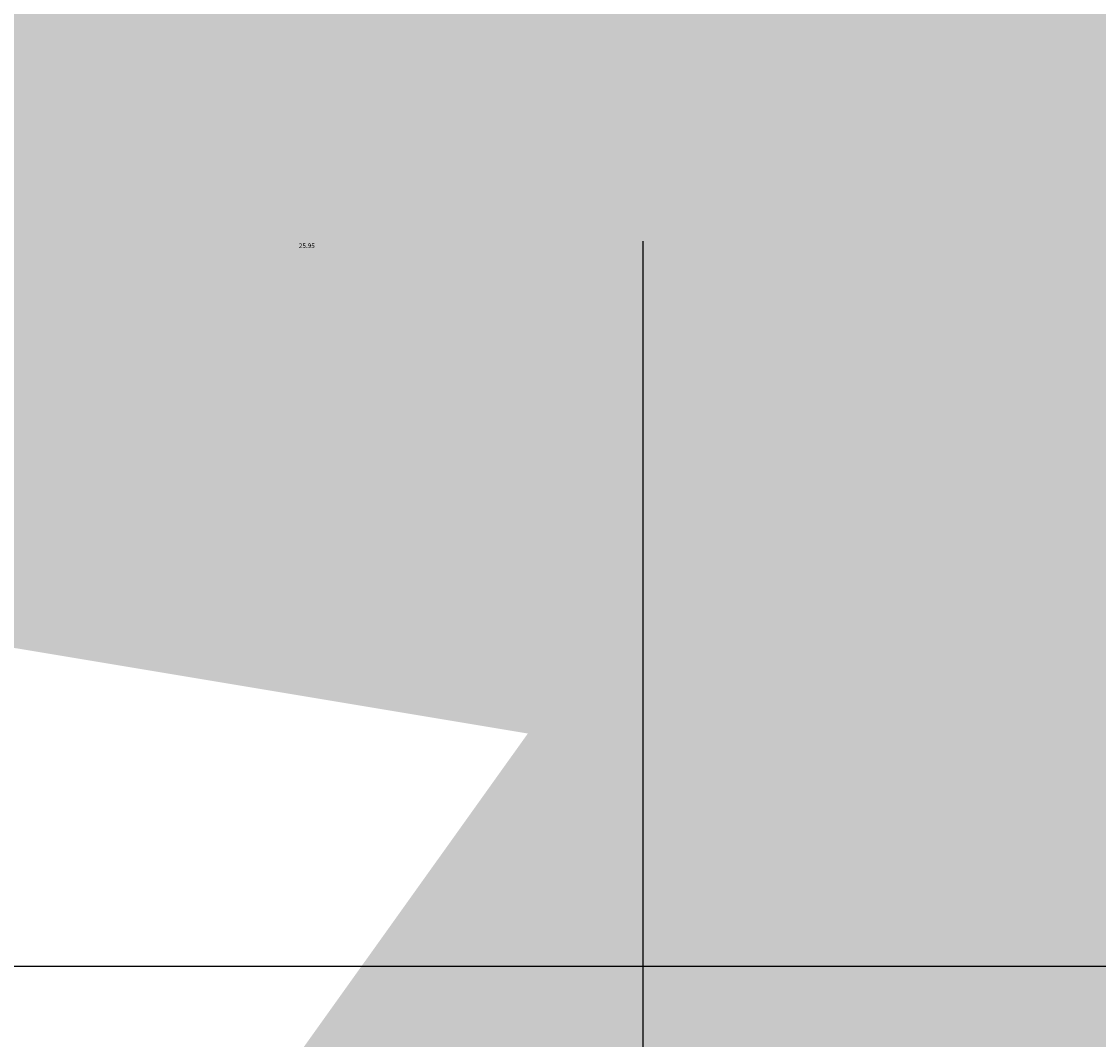
# Model space of a CAD drawing. Units: millimetres. Extents: x -22994 to 29398, y -19990 to 20176.
# Tile 119 of 135: x 204 to 245, y 174 to 213. Entities that reach past the tile are written whole.
import ezdxf

# ---------------------------------------------------------------- set-up
doc = ezdxf.new("R2010")
doc.units = ezdxf.units.MM
doc.header["$MEASUREMENT"] = 0
doc.layers.add('M-DIMS', color=2, linetype='Continuous', lineweight=18)
doc.styles.get("Standard").update_dxf_attribs({"font": 'arial.ttf'})
doc.dimstyles.get("Standard").update_dxf_attribs({"dimtxt": 0.18, "dimasz": 10000, "dimexe": 0.18, "dimexo": 0.0625, "dimgap": 0.09, "dimtad": 0, "dimtih": 1, "dimtoh": 1, "dimdec": 0, "dimzin": 0, "dimdsep": 46, "dimtxsty": 'Standard', "dimcen": 0.09, "dimadec": 0, "dimazin": 0, "dimtfac": 1, "dimtdec": 0, "dimtofl": 0, "dimtmove": 0, "dimatfit": 3, "dimfxl": 1, "dimtolj": 1, "dimtzin": 0, "dimlwd": 30, "dimarcsym": 0})

# ---------------------------------------------------------------- blocks, each defined once
blk = doc.blocks.new('*D2')
at = {"layer": 'Defpoints', "color": 0, "transparency": 16777216}
for p in [(6.677, 10.271), (290.852, 10.271), (290.852, -5.079)]:
    blk.add_point(p, dxfattribs=at)
at = {"layer": 'M-DIMS', "color": 0, "lineweight": -2, "transparency": 16777216}
for p, q in [((6.677, 10.209), (6.677, -5.259)), ((290.852, 10.209), (290.852, -5.259))]:
    blk.add_line(p, q, dxfattribs=at)
at = {"layer": 'M-DIMS', "color": 0, "lineweight": 30, "transparency": 16777216}
for p, q in [((-9993.323, -5.079), (-19993.323, -5.079)), ((10290.852, -5.079), (20290.852, -5.079))]:
    blk.add_line(p, q, dxfattribs=at)
at = {"layer": 'M-DIMS', "color": 0, "transparency": 16777216}
for points in [[(-9993.323, 1661.588), (-9993.323, -1671.745), (6.677, -5.079)], [(10290.852, 1661.588), (10290.852, -1671.745), (290.852, -5.079)]]:
    blk.add_solid(points, dxfattribs=at)
at = {"layer": 'M-DIMS', "color": 0, "transparency": 16777216, "insert": (148.765, -5.079), "char_height": 0.18, "attachment_point": 5}
blk.add_mtext('\\A1;284.2', dxfattribs=at)
blk = doc.blocks.new('*D3')
at = {"layer": 'Defpoints', "color": 0, "transparency": 16777216}
for p in [(110.265, 204.165), (110.265, 176.366), (95.833, 127.967)]:
    blk.add_point(p, dxfattribs=at)
at = {"layer": 'M-DIMS', "color": 0, "lineweight": 30, "transparency": 16777216}
for p, q in [((-9904.167, 204.165), (-19904.167, 204.165)), ((10110.265, 204.165), (20110.265, 204.165))]:
    blk.add_line(p, q, dxfattribs=at)
at = {"layer": 'M-DIMS', "color": 0, "lineweight": -2, "transparency": 16777216}
for p, q in [((95.833, 128.03), (95.833, 204.345)), ((110.265, 176.429), (110.265, 204.345))]:
    blk.add_line(p, q, dxfattribs=at)
at = {"layer": 'M-DIMS', "color": 0, "transparency": 16777216}
for points in [[(-9904.167, 1870.832), (-9904.167, -1462.501), (95.833, 204.165)], [(10110.265, 1870.832), (10110.265, -1462.501), (110.265, 204.165)]]:
    blk.add_solid(points, dxfattribs=at)
at = {"layer": 'M-DIMS', "color": 0, "transparency": 16777216, "insert": (103.049, 204.165), "char_height": 0.18, "attachment_point": 5}
blk.add_mtext('\\A1;14.432', dxfattribs=at)
blk = doc.blocks.new('*D4')
at = {"layer": 'Defpoints', "color": 0, "transparency": 16777216}
for p in [(116.265, 204.165), (110.265, 176.366), (116.265, 176.366)]:
    blk.add_point(p, dxfattribs=at)
at = {"layer": 'M-DIMS', "color": 0, "lineweight": 30, "transparency": 16777216}
for p, q in [((-9889.735, 204.165), (-19889.735, 204.165)), ((10116.265, 204.165), (20116.265, 204.165))]:
    blk.add_line(p, q, dxfattribs=at)
at = {"layer": 'M-DIMS', "color": 0, "lineweight": -2, "transparency": 16777216}
for p, q in [((110.265, 176.429), (110.265, 204.345)), ((116.265, 176.429), (116.265, 204.345))]:
    blk.add_line(p, q, dxfattribs=at)
at = {"layer": 'M-DIMS', "color": 0, "transparency": 16777216}
for points in [[(-9889.735, 1870.832), (-9889.735, -1462.501), (110.265, 204.165)], [(10116.265, 1870.832), (10116.265, -1462.501), (116.265, 204.165)]]:
    blk.add_solid(points, dxfattribs=at)
at = {"layer": 'M-DIMS', "color": 0, "transparency": 16777216, "insert": (113.265, 204.165), "char_height": 0.18, "attachment_point": 5}
blk.add_mtext('\\A1;6', dxfattribs=at)
blk = doc.blocks.new('*D5')
at = {"layer": 'Defpoints', "color": 0, "transparency": 16777216}
for p in [(181.265, 204.165), (116.265, 176.366), (181.265, 176.366)]:
    blk.add_point(p, dxfattribs=at)
at = {"layer": 'M-DIMS', "color": 0, "lineweight": 30, "transparency": 16777216}
for p, q in [((-9883.735, 204.165), (-19883.735, 204.165)), ((10181.265, 204.165), (20181.265, 204.165))]:
    blk.add_line(p, q, dxfattribs=at)
at = {"layer": 'M-DIMS', "color": 0, "lineweight": -2, "transparency": 16777216}
for p, q in [((116.265, 176.429), (116.265, 204.345)), ((181.265, 176.429), (181.265, 204.345))]:
    blk.add_line(p, q, dxfattribs=at)
at = {"layer": 'M-DIMS', "color": 0, "transparency": 16777216}
for points in [[(-9883.735, 1870.832), (-9883.735, -1462.501), (116.265, 204.165)], [(10181.265, 1870.832), (10181.265, -1462.501), (181.265, 204.165)]]:
    blk.add_solid(points, dxfattribs=at)
at = {"layer": 'M-DIMS', "color": 0, "transparency": 16777216, "insert": (148.765, 204.165), "char_height": 0.18, "attachment_point": 5}
blk.add_mtext('\\A1;65', dxfattribs=at)
blk = doc.blocks.new('*D6')
at = {"layer": 'Defpoints', "color": 0, "transparency": 16777216}
for p in [(187.265, 204.165), (181.265, 176.366), (187.265, 176.366)]:
    blk.add_point(p, dxfattribs=at)
at = {"layer": 'M-DIMS', "color": 0, "lineweight": 30, "transparency": 16777216}
for p, q in [((-9818.735, 204.165), (-19818.735, 204.165)), ((10187.265, 204.165), (20187.265, 204.165))]:
    blk.add_line(p, q, dxfattribs=at)
at = {"layer": 'M-DIMS', "color": 0, "lineweight": -2, "transparency": 16777216}
for p, q in [((181.265, 176.429), (181.265, 204.345)), ((187.265, 176.429), (187.265, 204.345))]:
    blk.add_line(p, q, dxfattribs=at)
at = {"layer": 'M-DIMS', "color": 0, "transparency": 16777216}
for points in [[(-9818.735, 1870.832), (-9818.735, -1462.501), (181.265, 204.165)], [(10187.265, 1870.832), (10187.265, -1462.501), (187.265, 204.165)]]:
    blk.add_solid(points, dxfattribs=at)
at = {"layer": 'M-DIMS', "color": 0, "transparency": 16777216, "insert": (184.265, 204.165), "char_height": 0.18, "attachment_point": 5}
blk.add_mtext('\\A1;6', dxfattribs=at)
blk = doc.blocks.new('*D7')
at = {"layer": 'Defpoints', "color": 0, "transparency": 16777216}
for p in [(201.697, 204.165), (187.265, 176.366), (201.697, 127.967)]:
    blk.add_point(p, dxfattribs=at)
at = {"layer": 'M-DIMS', "color": 0, "lineweight": 30, "transparency": 16777216}
for p, q in [((-9812.735, 204.165), (-19812.735, 204.165)), ((10201.697, 204.165), (20201.697, 204.165))]:
    blk.add_line(p, q, dxfattribs=at)
at = {"layer": 'M-DIMS', "color": 0, "lineweight": -2, "transparency": 16777216}
for p, q in [((187.265, 176.429), (187.265, 204.345)), ((201.697, 128.03), (201.697, 204.345))]:
    blk.add_line(p, q, dxfattribs=at)
at = {"layer": 'M-DIMS', "color": 0, "transparency": 16777216}
for points in [[(-9812.735, 1870.832), (-9812.735, -1462.501), (187.265, 204.165)], [(10201.697, 1870.832), (10201.697, -1462.501), (201.697, 204.165)]]:
    blk.add_solid(points, dxfattribs=at)
at = {"layer": 'M-DIMS', "color": 0, "transparency": 16777216, "insert": (194.481, 204.165), "char_height": 0.18, "attachment_point": 5}
blk.add_mtext('\\A1;14.432', dxfattribs=at)
blk = doc.blocks.new('*D8')
at = {"layer": 'Defpoints', "color": 0, "transparency": 16777216}
for p in [(227.648, 204.165), (227.648, 146.73), (201.697, 127.967)]:
    blk.add_point(p, dxfattribs=at)
at = {"layer": 'M-DIMS', "color": 0, "lineweight": 30, "transparency": 16777216}
for p, q in [((-9798.303, 204.165), (-19798.303, 204.165)), ((10227.648, 204.165), (20227.648, 204.165))]:
    blk.add_line(p, q, dxfattribs=at)
at = {"layer": 'M-DIMS', "color": 0, "lineweight": -2, "transparency": 16777216}
for p, q in [((201.697, 128.03), (201.697, 204.345)), ((227.648, 146.792), (227.648, 204.345))]:
    blk.add_line(p, q, dxfattribs=at)
at = {"layer": 'M-DIMS', "color": 0, "transparency": 16777216}
for points in [[(-9798.303, 1870.832), (-9798.303, -1462.501), (201.697, 204.165)], [(10227.648, 1870.832), (10227.648, -1462.501), (227.648, 204.165)]]:
    blk.add_solid(points, dxfattribs=at)
at = {"layer": 'M-DIMS', "color": 0, "transparency": 16777216, "insert": (214.673, 204.165), "char_height": 0.18, "attachment_point": 5}
blk.add_mtext('\\A1;25.95', dxfattribs=at)
blk = doc.blocks.new('*D9')
at = {"layer": 'Defpoints', "color": 0, "transparency": 16777216}
for p in [(187.265, 176.366), (306.202, 176.366), (290.852, 10.271)]:
    blk.add_point(p, dxfattribs=at)
at = {"layer": 'M-DIMS', "color": 0, "lineweight": 30, "transparency": 16777216}
for p, q in [((306.202, 10176.366), (306.202, 20176.366)), ((306.202, -9989.729), (306.202, -19989.729))]:
    blk.add_line(p, q, dxfattribs=at)
at = {"layer": 'M-DIMS', "color": 0, "lineweight": -2, "transparency": 16777216}
for p, q in [((187.327, 176.366), (306.382, 176.366)), ((290.915, 10.271), (306.382, 10.271))]:
    blk.add_line(p, q, dxfattribs=at)
at = {"layer": 'M-DIMS', "color": 0, "transparency": 16777216}
for points in [[(-1360.465, 10176.366), (1972.869, 10176.366), (306.202, 176.366)], [(-1360.465, -9989.729), (1972.869, -9989.729), (306.202, 10.271)]]:
    blk.add_solid(points, dxfattribs=at)
at = {"layer": 'M-DIMS', "color": 0, "transparency": 16777216, "insert": (306.202, 93.319), "char_height": 0.18, "attachment_point": 5}
blk.add_mtext('\\A1;166.1', dxfattribs=at)
blk = doc.blocks.new('*D10')
at = {"layer": 'Defpoints', "color": 0, "transparency": 16777216}
for p in [(125.65, 136.071), (133.346, 136.071), (133.346, -5.079)]:
    blk.add_point(p, dxfattribs=at)
at = {"layer": 'M-DIMS', "color": 0, "lineweight": -2, "transparency": 16777216}
for p, q in [((125.65, 136.009), (125.65, -5.259)), ((133.346, 136.009), (133.346, -5.259))]:
    blk.add_line(p, q, dxfattribs=at)
at = {"layer": 'M-DIMS', "color": 0, "lineweight": 30, "transparency": 16777216}
for p, q in [((-9874.35, -5.079), (-19874.35, -5.079)), ((10133.346, -5.079), (20133.346, -5.079))]:
    blk.add_line(p, q, dxfattribs=at)
at = {"layer": 'M-DIMS', "color": 0, "transparency": 16777216}
for points in [[(-9874.35, 1661.588), (-9874.35, -1671.745), (125.65, -5.079)], [(10133.346, 1661.588), (10133.346, -1671.745), (133.346, -5.079)]]:
    blk.add_solid(points, dxfattribs=at)
at = {"layer": 'M-DIMS', "color": 0, "transparency": 16777216, "insert": (129.498, -5.079), "char_height": 0.18, "attachment_point": 5}
blk.add_mtext('\\A1;7.696', dxfattribs=at)
blk = doc.blocks.new('*D11')
at = {"layer": 'Defpoints', "color": 0, "transparency": 16777216}
for p in [(133.346, 136.071), (135.65, 136.071), (135.65, -5.079)]:
    blk.add_point(p, dxfattribs=at)
at = {"layer": 'M-DIMS', "color": 0, "lineweight": -2, "transparency": 16777216}
for p, q in [((133.346, 136.009), (133.346, -5.259)), ((135.65, 136.009), (135.65, -5.259))]:
    blk.add_line(p, q, dxfattribs=at)
at = {"layer": 'M-DIMS', "color": 0, "lineweight": 30, "transparency": 16777216}
for p, q in [((-9866.654, -5.079), (-19866.654, -5.079)), ((10135.65, -5.079), (20135.65, -5.079))]:
    blk.add_line(p, q, dxfattribs=at)
at = {"layer": 'M-DIMS', "color": 0, "transparency": 16777216}
for points in [[(-9866.654, 1661.588), (-9866.654, -1671.745), (133.346, -5.079)], [(10135.65, 1661.588), (10135.65, -1671.745), (135.65, -5.079)]]:
    blk.add_solid(points, dxfattribs=at)
at = {"layer": 'M-DIMS', "color": 0, "transparency": 16777216, "insert": (134.498, -5.079), "char_height": 0.18, "attachment_point": 5}
blk.add_mtext('\\A1;2.304', dxfattribs=at)
blk = doc.blocks.new('*D12')
at = {"layer": 'Defpoints', "color": 0, "transparency": 16777216}
for p in [(135.65, 136.071), (145.65, 136.071), (145.65, -5.079)]:
    blk.add_point(p, dxfattribs=at)
at = {"layer": 'M-DIMS', "color": 0, "lineweight": -2, "transparency": 16777216}
for p, q in [((135.65, 136.009), (135.65, -5.259)), ((145.65, 136.009), (145.65, -5.259))]:
    blk.add_line(p, q, dxfattribs=at)
at = {"layer": 'M-DIMS', "color": 0, "lineweight": 30, "transparency": 16777216}
for p, q in [((-9864.35, -5.079), (-19864.35, -5.079)), ((10145.65, -5.079), (20145.65, -5.079))]:
    blk.add_line(p, q, dxfattribs=at)
at = {"layer": 'M-DIMS', "color": 0, "transparency": 16777216}
for points in [[(-9864.35, 1661.588), (-9864.35, -1671.745), (135.65, -5.079)], [(10145.65, 1661.588), (10145.65, -1671.745), (145.65, -5.079)]]:
    blk.add_solid(points, dxfattribs=at)
at = {"layer": 'M-DIMS', "color": 0, "transparency": 16777216, "insert": (140.65, -5.079), "char_height": 0.18, "attachment_point": 5}
blk.add_mtext('\\A1;10', dxfattribs=at)
blk = doc.blocks.new('*D13')
at = {"layer": 'Defpoints', "color": 0, "transparency": 16777216}
for p in [(145.65, 136.071), (155.65, 136.071), (155.65, -5.079)]:
    blk.add_point(p, dxfattribs=at)
at = {"layer": 'M-DIMS', "color": 0, "lineweight": -2, "transparency": 16777216}
for p, q in [((145.65, 136.009), (145.65, -5.259)), ((155.65, 136.009), (155.65, -5.259))]:
    blk.add_line(p, q, dxfattribs=at)
at = {"layer": 'M-DIMS', "color": 0, "lineweight": 30, "transparency": 16777216}
for p, q in [((-9854.35, -5.079), (-19854.35, -5.079)), ((10155.65, -5.079), (20155.65, -5.079))]:
    blk.add_line(p, q, dxfattribs=at)
at = {"layer": 'M-DIMS', "color": 0, "transparency": 16777216}
for points in [[(-9854.35, 1661.588), (-9854.35, -1671.745), (145.65, -5.079)], [(10155.65, 1661.588), (10155.65, -1671.745), (155.65, -5.079)]]:
    blk.add_solid(points, dxfattribs=at)
at = {"layer": 'M-DIMS', "color": 0, "transparency": 16777216, "insert": (150.65, -5.079), "char_height": 0.18, "attachment_point": 5}
blk.add_mtext('\\A1;10', dxfattribs=at)
blk = doc.blocks.new('*D14')
at = {"layer": 'Defpoints', "color": 0, "transparency": 16777216}
for p in [(155.65, 136.071), (165.65, 136.071), (165.65, -5.079)]:
    blk.add_point(p, dxfattribs=at)
at = {"layer": 'M-DIMS', "color": 0, "lineweight": -2, "transparency": 16777216}
for p, q in [((155.65, 136.009), (155.65, -5.259)), ((165.65, 136.009), (165.65, -5.259))]:
    blk.add_line(p, q, dxfattribs=at)
at = {"layer": 'M-DIMS', "color": 0, "lineweight": 30, "transparency": 16777216}
for p, q in [((-9844.35, -5.079), (-19844.35, -5.079)), ((10165.65, -5.079), (20165.65, -5.079))]:
    blk.add_line(p, q, dxfattribs=at)
at = {"layer": 'M-DIMS', "color": 0, "transparency": 16777216}
for points in [[(-9844.35, 1661.588), (-9844.35, -1671.745), (155.65, -5.079)], [(10165.65, 1661.588), (10165.65, -1671.745), (165.65, -5.079)]]:
    blk.add_solid(points, dxfattribs=at)
at = {"layer": 'M-DIMS', "color": 0, "transparency": 16777216, "insert": (160.65, -5.079), "char_height": 0.18, "attachment_point": 5}
blk.add_mtext('\\A1;10', dxfattribs=at)
blk = doc.blocks.new('*D15')
at = {"layer": 'Defpoints', "color": 0, "transparency": 16777216}
for p in [(173.346, 154.788), (173.346, 136.071), (306.202, 136.071)]:
    blk.add_point(p, dxfattribs=at)
at = {"layer": 'M-DIMS', "color": 0, "lineweight": 30, "transparency": 16777216}
for p, q in [((306.202, 10154.788), (306.202, 20154.788)), ((306.202, -9863.929), (306.202, -19863.929))]:
    blk.add_line(p, q, dxfattribs=at)
at = {"layer": 'M-DIMS', "color": 0, "lineweight": -2, "transparency": 16777216}
for p, q in [((173.408, 154.788), (306.382, 154.788)), ((173.408, 136.071), (306.382, 136.071))]:
    blk.add_line(p, q, dxfattribs=at)
at = {"layer": 'M-DIMS', "color": 0, "transparency": 16777216}
for points in [[(-1360.465, 10154.788), (1972.869, 10154.788), (306.202, 154.788)], [(-1360.465, -9863.929), (1972.869, -9863.929), (306.202, 136.071)]]:
    blk.add_solid(points, dxfattribs=at)
at = {"layer": 'M-DIMS', "color": 0, "transparency": 16777216, "insert": (306.202, 145.43), "char_height": 0.18, "attachment_point": 5}
blk.add_mtext('\\A1;18.717', dxfattribs=at)
blk = doc.blocks.new('*D16')
at = {"layer": 'Defpoints', "color": 0, "transparency": 16777216}
for p in [(120.17, 204.165), (110.466, 48.035), (120.17, 48.035)]:
    blk.add_point(p, dxfattribs=at)
at = {"layer": 'M-DIMS', "color": 0, "lineweight": 30, "transparency": 16777216}
for p, q in [((-9889.534, 204.165), (-19889.534, 204.165)), ((10120.17, 204.165), (20120.17, 204.165))]:
    blk.add_line(p, q, dxfattribs=at)
at = {"layer": 'M-DIMS', "color": 0, "lineweight": -2, "transparency": 16777216}
for p, q in [((110.466, 48.097), (110.466, 204.345)), ((120.17, 48.097), (120.17, 204.345))]:
    blk.add_line(p, q, dxfattribs=at)
at = {"layer": 'M-DIMS', "color": 0, "transparency": 16777216}
for points in [[(-9889.534, 1870.832), (-9889.534, -1462.501), (110.466, 204.165)], [(10120.17, 1870.832), (10120.17, -1462.501), (120.17, 204.165)]]:
    blk.add_solid(points, dxfattribs=at)
at = {"layer": 'M-DIMS', "color": 0, "transparency": 16777216, "insert": (115.318, 204.165), "char_height": 0.18, "attachment_point": 5}
blk.add_mtext('\\A1;9.704', dxfattribs=at)
blk = doc.blocks.new('*D17')
at = {"layer": 'Defpoints', "color": 0, "transparency": 16777216}
for p in [(126.17, 204.165), (120.17, 48.035), (126.17, 48.035)]:
    blk.add_point(p, dxfattribs=at)
at = {"layer": 'M-DIMS', "color": 0, "lineweight": 30, "transparency": 16777216}
for p, q in [((-9879.83, 204.165), (-19879.83, 204.165)), ((10126.17, 204.165), (20126.17, 204.165))]:
    blk.add_line(p, q, dxfattribs=at)
at = {"layer": 'M-DIMS', "color": 0, "lineweight": -2, "transparency": 16777216}
for p, q in [((120.17, 48.097), (120.17, 204.345)), ((126.17, 48.097), (126.17, 204.345))]:
    blk.add_line(p, q, dxfattribs=at)
at = {"layer": 'M-DIMS', "color": 0, "transparency": 16777216}
for points in [[(-9879.83, 1870.832), (-9879.83, -1462.501), (120.17, 204.165)], [(10126.17, 1870.832), (10126.17, -1462.501), (126.17, 204.165)]]:
    blk.add_solid(points, dxfattribs=at)
at = {"layer": 'M-DIMS', "color": 0, "transparency": 16777216, "insert": (123.17, 204.165), "char_height": 0.18, "attachment_point": 5}
blk.add_mtext('\\A1;6', dxfattribs=at)
blk = doc.blocks.new('*D18')
at = {"layer": 'Defpoints', "color": 0, "transparency": 16777216}
for p in [(132.17, 204.165), (126.17, 48.035), (132.17, 48.035)]:
    blk.add_point(p, dxfattribs=at)
at = {"layer": 'M-DIMS', "color": 0, "lineweight": 30, "transparency": 16777216}
for p, q in [((-9873.83, 204.165), (-19873.83, 204.165)), ((10132.17, 204.165), (20132.17, 204.165))]:
    blk.add_line(p, q, dxfattribs=at)
at = {"layer": 'M-DIMS', "color": 0, "lineweight": -2, "transparency": 16777216}
for p, q in [((126.17, 48.097), (126.17, 204.345)), ((132.17, 48.097), (132.17, 204.345))]:
    blk.add_line(p, q, dxfattribs=at)
at = {"layer": 'M-DIMS', "color": 0, "transparency": 16777216}
for points in [[(-9873.83, 1870.832), (-9873.83, -1462.501), (126.17, 204.165)], [(10132.17, 1870.832), (10132.17, -1462.501), (132.17, 204.165)]]:
    blk.add_solid(points, dxfattribs=at)
at = {"layer": 'M-DIMS', "color": 0, "transparency": 16777216, "insert": (129.17, 204.165), "char_height": 0.18, "attachment_point": 5}
blk.add_mtext('\\A1;6', dxfattribs=at)
blk = doc.blocks.new('*D19')
at = {"layer": 'Defpoints', "color": 0, "transparency": 16777216}
for p in [(138.17, 204.165), (132.17, 48.035), (138.17, 48.035)]:
    blk.add_point(p, dxfattribs=at)
at = {"layer": 'M-DIMS', "color": 0, "lineweight": 30, "transparency": 16777216}
for p, q in [((-9867.83, 204.165), (-19867.83, 204.165)), ((10138.17, 204.165), (20138.17, 204.165))]:
    blk.add_line(p, q, dxfattribs=at)
at = {"layer": 'M-DIMS', "color": 0, "lineweight": -2, "transparency": 16777216}
for p, q in [((132.17, 48.097), (132.17, 204.345)), ((138.17, 48.097), (138.17, 204.345))]:
    blk.add_line(p, q, dxfattribs=at)
at = {"layer": 'M-DIMS', "color": 0, "transparency": 16777216}
for points in [[(-9867.83, 1870.832), (-9867.83, -1462.501), (132.17, 204.165)], [(10138.17, 1870.832), (10138.17, -1462.501), (138.17, 204.165)]]:
    blk.add_solid(points, dxfattribs=at)
at = {"layer": 'M-DIMS', "color": 0, "transparency": 16777216, "insert": (135.17, 204.165), "char_height": 0.18, "attachment_point": 5}
blk.add_mtext('\\A1;6', dxfattribs=at)
blk = doc.blocks.new('*D20')
at = {"layer": 'Defpoints', "color": 0, "transparency": 16777216}
for p in [(144.17, 204.165), (138.17, 48.035), (144.17, 48.035)]:
    blk.add_point(p, dxfattribs=at)
at = {"layer": 'M-DIMS', "color": 0, "lineweight": 30, "transparency": 16777216}
for p, q in [((-9861.83, 204.165), (-19861.83, 204.165)), ((10144.17, 204.165), (20144.17, 204.165))]:
    blk.add_line(p, q, dxfattribs=at)
at = {"layer": 'M-DIMS', "color": 0, "lineweight": -2, "transparency": 16777216}
for p, q in [((138.17, 48.097), (138.17, 204.345)), ((144.17, 48.097), (144.17, 204.345))]:
    blk.add_line(p, q, dxfattribs=at)
at = {"layer": 'M-DIMS', "color": 0, "transparency": 16777216}
for points in [[(-9861.83, 1870.832), (-9861.83, -1462.501), (138.17, 204.165)], [(10144.17, 1870.832), (10144.17, -1462.501), (144.17, 204.165)]]:
    blk.add_solid(points, dxfattribs=at)
at = {"layer": 'M-DIMS', "color": 0, "transparency": 16777216, "insert": (141.17, 204.165), "char_height": 0.18, "attachment_point": 5}
blk.add_mtext('\\A1;6', dxfattribs=at)
blk = doc.blocks.new('*D21')
at = {"layer": 'Defpoints', "color": 0, "transparency": 16777216}
for p in [(149.116, 204.165), (144.17, 48.035), (149.116, 48.035)]:
    blk.add_point(p, dxfattribs=at)
at = {"layer": 'M-DIMS', "color": 0, "lineweight": 30, "transparency": 16777216}
for p, q in [((-9855.83, 204.165), (-19855.83, 204.165)), ((10149.116, 204.165), (20149.116, 204.165))]:
    blk.add_line(p, q, dxfattribs=at)
at = {"layer": 'M-DIMS', "color": 0, "lineweight": -2, "transparency": 16777216}
for p, q in [((144.17, 48.097), (144.17, 204.345)), ((149.116, 48.097), (149.116, 204.345))]:
    blk.add_line(p, q, dxfattribs=at)
at = {"layer": 'M-DIMS', "color": 0, "transparency": 16777216}
for points in [[(-9855.83, 1870.832), (-9855.83, -1462.501), (144.17, 204.165)], [(10149.116, 1870.832), (10149.116, -1462.501), (149.116, 204.165)]]:
    blk.add_solid(points, dxfattribs=at)
at = {"layer": 'M-DIMS', "color": 0, "transparency": 16777216, "insert": (146.643, 204.165), "char_height": 0.18, "attachment_point": 5}
blk.add_mtext('\\A1;4.945', dxfattribs=at)
blk = doc.blocks.new('*D22')
at = {"layer": 'Defpoints', "color": 0, "transparency": 16777216}
for p in [(149.116, 30.99), (155.116, 30.99), (155.116, -5.079)]:
    blk.add_point(p, dxfattribs=at)
at = {"layer": 'M-DIMS', "color": 0, "lineweight": -2, "transparency": 16777216}
for p, q in [((149.116, 30.927), (149.116, -5.259)), ((155.116, 30.927), (155.116, -5.259))]:
    blk.add_line(p, q, dxfattribs=at)
at = {"layer": 'M-DIMS', "color": 0, "lineweight": 30, "transparency": 16777216}
for p, q in [((-9850.884, -5.079), (-19850.884, -5.079)), ((10155.116, -5.079), (20155.116, -5.079))]:
    blk.add_line(p, q, dxfattribs=at)
at = {"layer": 'M-DIMS', "color": 0, "transparency": 16777216}
for points in [[(-9850.884, 1661.588), (-9850.884, -1671.745), (149.116, -5.079)], [(10155.116, 1661.588), (10155.116, -1671.745), (155.116, -5.079)]]:
    blk.add_solid(points, dxfattribs=at)
at = {"layer": 'M-DIMS', "color": 0, "transparency": 16777216, "insert": (152.116, -5.079), "char_height": 0.18, "attachment_point": 5}
blk.add_mtext('\\A1;6', dxfattribs=at)
blk = doc.blocks.new('*D23')
at = {"layer": 'Defpoints', "color": 0, "transparency": 16777216}
for p in [(155.116, 30.99), (161.116, 30.99), (161.116, -5.079)]:
    blk.add_point(p, dxfattribs=at)
at = {"layer": 'M-DIMS', "color": 0, "lineweight": -2, "transparency": 16777216}
for p, q in [((155.116, 30.927), (155.116, -5.259)), ((161.116, 30.927), (161.116, -5.259))]:
    blk.add_line(p, q, dxfattribs=at)
at = {"layer": 'M-DIMS', "color": 0, "lineweight": 30, "transparency": 16777216}
for p, q in [((-9844.884, -5.079), (-19844.884, -5.079)), ((10161.116, -5.079), (20161.116, -5.079))]:
    blk.add_line(p, q, dxfattribs=at)
at = {"layer": 'M-DIMS', "color": 0, "transparency": 16777216}
for points in [[(-9844.884, 1661.588), (-9844.884, -1671.745), (155.116, -5.079)], [(10161.116, 1661.588), (10161.116, -1671.745), (161.116, -5.079)]]:
    blk.add_solid(points, dxfattribs=at)
at = {"layer": 'M-DIMS', "color": 0, "transparency": 16777216, "insert": (158.116, -5.079), "char_height": 0.18, "attachment_point": 5}
blk.add_mtext('\\A1;6', dxfattribs=at)
blk = doc.blocks.new('*D24')
at = {"layer": 'Defpoints', "color": 0, "transparency": 16777216}
for p in [(161.116, 30.99), (166.439, 30.99), (166.439, -5.079)]:
    blk.add_point(p, dxfattribs=at)
at = {"layer": 'M-DIMS', "color": 0, "lineweight": -2, "transparency": 16777216}
for p, q in [((161.116, 30.927), (161.116, -5.259)), ((166.439, 30.927), (166.439, -5.259))]:
    blk.add_line(p, q, dxfattribs=at)
at = {"layer": 'M-DIMS', "color": 0, "lineweight": 30, "transparency": 16777216}
for p, q in [((-9838.884, -5.079), (-19838.884, -5.079)), ((10166.439, -5.079), (20166.439, -5.079))]:
    blk.add_line(p, q, dxfattribs=at)
at = {"layer": 'M-DIMS', "color": 0, "transparency": 16777216}
for points in [[(-9838.884, 1661.588), (-9838.884, -1671.745), (161.116, -5.079)], [(10166.439, 1661.588), (10166.439, -1671.745), (166.439, -5.079)]]:
    blk.add_solid(points, dxfattribs=at)
at = {"layer": 'M-DIMS', "color": 0, "transparency": 16777216, "insert": (163.777, -5.079), "char_height": 0.18, "attachment_point": 5}
blk.add_mtext('\\A1;5.323', dxfattribs=at)
blk = doc.blocks.new('*D25')
at = {"layer": 'Defpoints', "color": 0, "transparency": 16777216}
for p in [(166.439, 30.99), (172.439, 30.99), (172.439, -5.079)]:
    blk.add_point(p, dxfattribs=at)
at = {"layer": 'M-DIMS', "color": 0, "lineweight": -2, "transparency": 16777216}
for p, q in [((166.439, 30.927), (166.439, -5.259)), ((172.439, 30.927), (172.439, -5.259))]:
    blk.add_line(p, q, dxfattribs=at)
at = {"layer": 'M-DIMS', "color": 0, "lineweight": 30, "transparency": 16777216}
for p, q in [((-9833.561, -5.079), (-19833.561, -5.079)), ((10172.439, -5.079), (20172.439, -5.079))]:
    blk.add_line(p, q, dxfattribs=at)
at = {"layer": 'M-DIMS', "color": 0, "transparency": 16777216}
for points in [[(-9833.561, 1661.588), (-9833.561, -1671.745), (166.439, -5.079)], [(10172.439, 1661.588), (10172.439, -1671.745), (172.439, -5.079)]]:
    blk.add_solid(points, dxfattribs=at)
at = {"layer": 'M-DIMS', "color": 0, "transparency": 16777216, "insert": (169.439, -5.079), "char_height": 0.18, "attachment_point": 5}
blk.add_mtext('\\A1;6', dxfattribs=at)
blk = doc.blocks.new('*D26')
at = {"layer": 'Defpoints', "color": 0, "transparency": 16777216}
for p in [(172.439, 30.99), (178.439, 30.99), (178.439, -5.079)]:
    blk.add_point(p, dxfattribs=at)
at = {"layer": 'M-DIMS', "color": 0, "lineweight": -2, "transparency": 16777216}
for p, q in [((172.439, 30.927), (172.439, -5.259)), ((178.439, 30.927), (178.439, -5.259))]:
    blk.add_line(p, q, dxfattribs=at)
at = {"layer": 'M-DIMS', "color": 0, "lineweight": 30, "transparency": 16777216}
for p, q in [((-9827.561, -5.079), (-19827.561, -5.079)), ((10178.439, -5.079), (20178.439, -5.079))]:
    blk.add_line(p, q, dxfattribs=at)
at = {"layer": 'M-DIMS', "color": 0, "transparency": 16777216}
for points in [[(-9827.561, 1661.588), (-9827.561, -1671.745), (172.439, -5.079)], [(10178.439, 1661.588), (10178.439, -1671.745), (178.439, -5.079)]]:
    blk.add_solid(points, dxfattribs=at)
at = {"layer": 'M-DIMS', "color": 0, "transparency": 16777216, "insert": (175.439, -5.079), "char_height": 0.18, "attachment_point": 5}
blk.add_mtext('\\A1;6', dxfattribs=at)
blk = doc.blocks.new('*D27')
at = {"layer": 'Defpoints', "color": 0, "transparency": 16777216}
for p in [(178.439, 30.99), (188.117, 30.99), (188.117, -5.079)]:
    blk.add_point(p, dxfattribs=at)
at = {"layer": 'M-DIMS', "color": 0, "lineweight": -2, "transparency": 16777216}
for p, q in [((178.439, 30.927), (178.439, -5.259)), ((188.117, 30.927), (188.117, -5.259))]:
    blk.add_line(p, q, dxfattribs=at)
at = {"layer": 'M-DIMS', "color": 0, "lineweight": 30, "transparency": 16777216}
for p, q in [((-9821.561, -5.079), (-19821.561, -5.079)), ((10188.117, -5.079), (20188.117, -5.079))]:
    blk.add_line(p, q, dxfattribs=at)
at = {"layer": 'M-DIMS', "color": 0, "transparency": 16777216}
for points in [[(-9821.561, 1661.588), (-9821.561, -1671.745), (178.439, -5.079)], [(10188.117, 1661.588), (10188.117, -1671.745), (188.117, -5.079)]]:
    blk.add_solid(points, dxfattribs=at)
at = {"layer": 'M-DIMS', "color": 0, "transparency": 16777216, "insert": (183.278, -5.079), "char_height": 0.18, "attachment_point": 5}
blk.add_mtext('\\A1;9.679', dxfattribs=at)
blk = doc.blocks.new('*D28')
at = {"layer": 'Defpoints', "color": 0, "transparency": 16777216}
for p in [(188.117, 48.035), (306.202, 48.035), (188.117, 30.99)]:
    blk.add_point(p, dxfattribs=at)
at = {"layer": 'M-DIMS', "color": 0, "lineweight": 30, "transparency": 16777216}
for p, q in [((306.202, 10048.035), (306.202, 20048.035)), ((306.202, -9969.01), (306.202, -19969.01))]:
    blk.add_line(p, q, dxfattribs=at)
at = {"layer": 'M-DIMS', "color": 0, "lineweight": -2, "transparency": 16777216}
for p, q in [((188.18, 48.035), (306.382, 48.035)), ((188.18, 30.99), (306.382, 30.99))]:
    blk.add_line(p, q, dxfattribs=at)
at = {"layer": 'M-DIMS', "color": 0, "transparency": 16777216}
for points in [[(-1360.465, 10048.035), (1972.869, 10048.035), (306.202, 48.035)], [(-1360.465, -9969.01), (1972.869, -9969.01), (306.202, 30.99)]]:
    blk.add_solid(points, dxfattribs=at)
at = {"layer": 'M-DIMS', "color": 0, "transparency": 16777216, "insert": (306.202, 39.512), "char_height": 0.18, "attachment_point": 5}
blk.add_mtext('\\A1;17.045', dxfattribs=at)
blk = doc.blocks.new('*D29')
at = {"layer": 'Defpoints', "color": 0, "transparency": 16777216}
for p in [(36.801, 80.045), (64.03, 80.045)]:
    blk.add_point(p, dxfattribs=at)
at = {"layer": 'M-DIMS', "color": 0, "lineweight": -2, "transparency": 16777216}
for p, q in [((50.325, 80.045), (50.505, 80.045)), ((50.415, 79.955), (50.415, 80.135))]:
    blk.add_line(p, q, dxfattribs=at)
at = {"layer": 'M-DIMS', "color": 0, "lineweight": 30, "transparency": 16777216}
blk.add_line((20064.03, 80.03), (10064.03, 80.038), dxfattribs=at)
at = {"layer": 'M-DIMS', "color": 0, "transparency": 16777216}
blk.add_solid([(10064.031, 1746.704), (10064.028, -1586.629), (64.03, 80.045)], dxfattribs=at)
at = {"layer": 'M-DIMS', "color": 0, "transparency": 16777216, "insert": (20064.521, 80.03), "char_height": 0.18, "attachment_point": 5}
blk.add_mtext('\\A1;∅27.23', dxfattribs=at)
blk = doc.blocks.new('*D30')
at = {"layer": 'Defpoints', "color": 0, "transparency": 16777216}
for p in [(216.315, 146.729), (238.982, 146.73)]:
    blk.add_point(p, dxfattribs=at)
at = {"layer": 'M-DIMS', "color": 0, "lineweight": 30, "transparency": 16777216}
blk.add_line((20238.982, 147.496), (10238.982, 147.113), dxfattribs=at)
at = {"layer": 'M-DIMS', "color": 0, "lineweight": -2, "transparency": 16777216}
for p, q in [((227.558, 146.73), (227.738, 146.73)), ((227.648, 146.64), (227.648, 146.82))]:
    blk.add_line(p, q, dxfattribs=at)
at = {"layer": 'M-DIMS', "color": 0, "transparency": 16777216}
blk.add_solid([(10238.918, 1813.78), (10239.046, -1519.554), (238.982, 146.73)], dxfattribs=at)
at = {"layer": 'M-DIMS', "color": 0, "transparency": 16777216, "insert": (20239.544, 147.496), "char_height": 0.18, "attachment_point": 5}
blk.add_mtext('\\A1;∅22.667', dxfattribs=at)
blk = doc.blocks.new('*D31')
at = {"layer": 'Defpoints', "color": 0, "transparency": 16777216}
for p in [(223.164, 146.729), (232.133, 146.73)]:
    blk.add_point(p, dxfattribs=at)
at = {"layer": 'M-DIMS', "color": 0, "lineweight": 30, "transparency": 16777216}
blk.add_line((20232.133, 148.666), (10232.133, 147.698), dxfattribs=at)
at = {"layer": 'M-DIMS', "color": 0, "lineweight": -2, "transparency": 16777216}
for p, q in [((227.558, 146.73), (227.738, 146.73)), ((227.648, 146.64), (227.648, 146.82))]:
    blk.add_line(p, q, dxfattribs=at)
at = {"layer": 'M-DIMS', "color": 0, "transparency": 16777216}
blk.add_solid([(10231.971, 1814.364), (10232.294, -1518.969), (232.133, 146.73)], dxfattribs=at)
at = {"layer": 'M-DIMS', "color": 0, "transparency": 16777216, "insert": (20232.625, 148.666), "char_height": 0.18, "attachment_point": 5}
blk.add_mtext('\\A1;∅8.969', dxfattribs=at)
blk = doc.blocks.new('*D34')
at = {"layer": 'Defpoints', "color": 0, "transparency": 16777216}
for p in [(178.58, 122.895), (176.812, 121.128)]:
    blk.add_point(p, dxfattribs=at)
at = {"layer": 'M-DIMS', "color": 0, "lineweight": 30, "transparency": 16777216}
for p, q in [((14322.436, 14263.311), (7250.508, 7193.103)), ((24322.436, 14263.311), (14322.436, 14263.311))]:
    blk.add_line(p, q, dxfattribs=at)
at = {"layer": 'M-DIMS', "color": 0, "lineweight": -2, "transparency": 16777216}
for p, q in [((176.722, 121.128), (176.902, 121.128)), ((176.812, 121.038), (176.812, 121.218))]:
    blk.add_line(p, q, dxfattribs=at)
at = {"layer": 'M-DIMS', "color": 0, "transparency": 16777216}
blk.add_solid([(6072.14, 8371.758), (8428.876, 6014.448), (178.58, 122.895)], dxfattribs=at)
at = {"layer": 'M-DIMS', "color": 0, "transparency": 16777216, "insert": (24322.97, 14263.311), "char_height": 0.18, "attachment_point": 5}
blk.add_mtext('\\A1;6X R2.5', dxfattribs=at)
blk = doc.blocks.new('*D36')
at = {"layer": 'Defpoints', "color": 0, "transparency": 16777216}
for p in [(46.39, 31.303), (46.387, 26.593)]:
    blk.add_point(p, dxfattribs=at)
at = {"layer": 'M-DIMS', "color": 0, "lineweight": 30, "transparency": 16777216}
for p, q in [((57.15, 20031.301), (51.77, 10031.302)), ((10057.15, 20031.301), (57.15, 20031.301))]:
    blk.add_line(p, q, dxfattribs=at)
at = {"layer": 'M-DIMS', "color": 0, "lineweight": -2, "transparency": 16777216}
for p, q in [((46.299, 28.948), (46.479, 28.948)), ((46.389, 28.858), (46.389, 29.038))]:
    blk.add_line(p, q, dxfattribs=at)
at = {"layer": 'M-DIMS', "color": 0, "transparency": 16777216}
blk.add_solid([(-1614.896, 10032.199), (1718.436, 10030.405), (46.39, 31.303)], dxfattribs=at)
at = {"layer": 'M-DIMS', "color": 0, "transparency": 16777216, "insert": (10057.554, 20031.301), "char_height": 0.18, "attachment_point": 5}
blk.add_mtext('\\A1;∅4.71', dxfattribs=at)
blk = doc.blocks.new('*D37')
at = {"layer": 'Defpoints', "color": 0, "transparency": 16777216}
for p in [(54.834, 118.615), (59.494, 118.614)]:
    blk.add_point(p, dxfattribs=at)
at = {"layer": 'M-DIMS', "color": 0, "lineweight": -2, "transparency": 16777216}
for p, q in [((57.074, 118.614), (57.254, 118.614)), ((57.164, 118.524), (57.164, 118.704))]:
    blk.add_line(p, q, dxfattribs=at)
at = {"layer": 'M-DIMS', "color": 0, "lineweight": 30, "transparency": 16777216}
blk.add_line((20059.493, 116.253), (10059.494, 117.434), dxfattribs=at)
at = {"layer": 'M-DIMS', "color": 0, "transparency": 16777216}
blk.add_solid([(10059.69, 1784.1), (10059.297, -1549.233), (59.494, 118.614)], dxfattribs=at)
at = {"layer": 'M-DIMS', "color": 0, "transparency": 16777216, "insert": (20059.985, 116.253), "char_height": 0.18, "attachment_point": 5}
blk.add_mtext('\\A1;∅4.659', dxfattribs=at)

msp = doc.modelspace()

# ---------------------------------------------------------------- dimensions: what is measured, and where the dimension line sits
at = {"layer": 'M-DIMS'}
for base, p1, p2, override, picture, middle in [((306.202, 176.3662), (290.852, 10.2713), (187.2647, 176.3662), {"dimdec": 1, "dimlfac": 1, "dimrnd": 0, "dimzin": 0, "dimdsep": 46, "dimlunit": 2}, '*D9', (306.202, 93.3187)), ((306.202, 136.0713), (173.3459, 154.788), (173.3459, 136.0713), {"dimdec": 3, "dimlfac": 1, "dimrnd": 0, "dimzin": 0, "dimdsep": 46, "dimlunit": 2}, '*D15', (306.202, 145.4297)), ((306.202, 48.0349), (188.1175, 30.9895), (188.1175, 48.0349), {"dimdec": 3, "dimlfac": 1, "dimrnd": 0, "dimzin": 0, "dimdsep": 46, "dimlunit": 2}, '*D28', (306.202, 39.5122))]:
    dim = msp.add_linear_dim(base=base, p1=p1, p2=p2, angle=90, dimstyle='Standard', override=override, dxfattribs=at)
    dim.commit()
    dim.dimension.update_dxf_attribs({"geometry": picture, "text_midpoint": middle})
for p1, p2, override, picture, middle in [((46.3875, 26.5934), (46.39, 31.3035), {"dimdec": 2, "dimlfac": 1, "dimrnd": 0, "dimzin": 0, "dimdsep": 46, "dimlunit": 2}, '*D36', (10057.5542, 20031.3006)), ((223.1641, 146.7291), (232.1328, 146.73), {"dimdec": 3, "dimlfac": 1, "dimrnd": 0, "dimzin": 0, "dimdsep": 46, "dimlunit": 2}, '*D31', (20232.1327, 148.6656)), ((216.3148, 146.7291), (238.9821, 146.73), {"dimdec": 3, "dimlfac": 1, "dimrnd": 0, "dimzin": 0, "dimdsep": 46, "dimlunit": 2}, '*D30', (20238.9821, 147.4959))]:
    dim = msp.add_diameter_dim_2p(p1=p1, p2=p2, dimstyle='Standard', override=override, dxfattribs=at)
    dim.commit()
    dim.dimension.update_dxf_attribs({"geometry": picture, "text_midpoint": middle, "dimtype": 163})
dim = msp.add_radius_dim(center=(176.8123, 121.1277), mpoint=(178.5802, 122.8952), text='6X <>', dimstyle='Standard', override={"dimdec": 1, "dimlfac": 1, "dimrnd": 0, "dimzin": 0, "dimdsep": 46, "dimlunit": 2}, dxfattribs=at)
dim.commit()
dim.dimension.update_dxf_attribs({"geometry": '*D34', "text_midpoint": (24322.9703, 14263.3108)})
for base, p1, p2, override, picture, middle in [((110.2647, 204.1654), (95.8327, 127.967), (110.2647, 176.3662), {"dimdec": 3, "dimlfac": 1, "dimrnd": 0, "dimzin": 0, "dimdsep": 46, "dimlunit": 2}, '*D3', (103.0487, 204.1654)), ((116.2647, 204.1654), (110.2647, 176.3662), (116.2647, 176.3662), {"dimdec": 0, "dimlfac": 1, "dimrnd": 0, "dimzin": 0, "dimdsep": 46, "dimlunit": 2}, '*D4', (113.2647, 204.1654)), ((120.1702, 204.1654), (110.4658, 48.0349), (120.1702, 48.0349), {"dimdec": 3, "dimlfac": 1, "dimrnd": 0, "dimzin": 0, "dimdsep": 46, "dimlunit": 2}, '*D16', (115.318, 204.1654)), ((181.2647, 204.1654), (116.2647, 176.3662), (181.2647, 176.3662), {"dimdec": 0, "dimlfac": 1, "dimrnd": 0, "dimzin": 0, "dimdsep": 46, "dimlunit": 2}, '*D5', (148.7647, 204.1654)), ((126.1702, 204.1654), (120.1702, 48.0349), (126.1702, 48.0349), {"dimdec": 0, "dimlfac": 1, "dimrnd": 0, "dimzin": 0, "dimdsep": 46, "dimlunit": 2}, '*D17', (123.1702, 204.1654)), ((132.1702, 204.1654), (126.1702, 48.0349), (132.1702, 48.0349), {"dimdec": 0, "dimlfac": 1, "dimrnd": 0, "dimzin": 0, "dimdsep": 46, "dimlunit": 2}, '*D18', (129.1702, 204.1654)), ((138.1702, 204.1654), (132.1702, 48.0349), (138.1702, 48.0349), {"dimdec": 0, "dimlfac": 1, "dimrnd": 0, "dimzin": 0, "dimdsep": 46, "dimlunit": 2}, '*D19', (135.1702, 204.1654)), ((144.1702, 204.1654), (138.1702, 48.0349), (144.1702, 48.0349), {"dimdec": 0, "dimlfac": 1, "dimrnd": 0, "dimzin": 0, "dimdsep": 46, "dimlunit": 2}, '*D20', (141.1702, 204.1654)), ((149.11567, 204.16539), (144.17023, 48.03494), (149.11567, 48.03494), {"dimdec": 3, "dimlfac": 1, "dimrnd": 0, "dimzin": 0, "dimdsep": 46, "dimlunit": 2}, '*D21', (146.64295, 204.16539)), ((187.2647, 204.1654), (181.2647, 176.3662), (187.2647, 176.3662), {"dimdec": 0, "dimlfac": 1, "dimrnd": 0, "dimzin": 0, "dimdsep": 46, "dimlunit": 2}, '*D6', (184.2647, 204.1654)), ((201.6967, 204.1654), (187.2647, 176.3662), (201.6967, 127.967), {"dimdec": 3, "dimlfac": 1, "dimrnd": 0, "dimzin": 0, "dimdsep": 46, "dimlunit": 2}, '*D7', (194.4807, 204.1654)), ((227.6485, 204.1654), (201.6967, 127.967), (227.6485, 146.7296), {"dimdec": 2, "dimlfac": 1, "dimrnd": 0, "dimzin": 0, "dimdsep": 46, "dimlunit": 2}, '*D8', (214.6726, 204.1654)), ((290.852, -5.0787), (6.6773, 10.2713), (290.852, 10.2713), {"dimdec": 1, "dimlfac": 1, "dimrnd": 0, "dimzin": 0, "dimdsep": 46, "dimlunit": 2}, '*D2', (148.7647, -5.0787)), ((133.3459, -5.0787), (125.6498, 136.0713), (133.3459, 136.0713), {"dimdec": 3, "dimlfac": 1, "dimrnd": 0, "dimzin": 0, "dimdsep": 46, "dimlunit": 2}, '*D10', (129.4978, -5.0787)), ((135.6498, -5.0787), (133.3459, 136.0713), (135.6498, 136.0713), {"dimdec": 3, "dimlfac": 1, "dimrnd": 0, "dimzin": 0, "dimdsep": 46, "dimlunit": 2}, '*D11', (134.4978, -5.0787)), ((145.6498, -5.0787), (135.6498, 136.0713), (145.6498, 136.0713), {"dimdec": 0, "dimlfac": 1, "dimrnd": 0, "dimzin": 0, "dimdsep": 46, "dimlunit": 2}, '*D12', (140.6498, -5.0787)), ((155.6498, -5.0787), (145.6498, 136.0713), (155.6498, 136.0713), {"dimdec": 0, "dimlfac": 1, "dimrnd": 0, "dimzin": 0, "dimdsep": 46, "dimlunit": 2}, '*D13', (150.6498, -5.0787)), ((155.1157, -5.0787), (149.1157, 30.9895), (155.1157, 30.9895), {"dimdec": 0, "dimlfac": 1, "dimrnd": 0, "dimzin": 0, "dimdsep": 46, "dimlunit": 2}, '*D22', (152.1157, -5.0787)), ((161.1157, -5.0787), (155.1157, 30.9895), (161.1157, 30.9895), {"dimdec": 0, "dimlfac": 1, "dimrnd": 0, "dimzin": 0, "dimdsep": 46, "dimlunit": 2}, '*D23', (158.1157, -5.0787)), ((165.6498, -5.0787), (155.6498, 136.0713), (165.6498, 136.0713), {"dimdec": 0, "dimlfac": 1, "dimrnd": 0, "dimzin": 0, "dimdsep": 46, "dimlunit": 2}, '*D14', (160.6498, -5.0787)), ((166.4387, -5.0787), (161.1157, 30.9895), (166.4387, 30.9895), {"dimdec": 3, "dimlfac": 1, "dimrnd": 0, "dimzin": 0, "dimdsep": 46, "dimlunit": 2}, '*D24', (163.7772, -5.0787)), ((172.4387, -5.0787), (166.4387, 30.9895), (172.4387, 30.9895), {"dimdec": 0, "dimlfac": 1, "dimrnd": 0, "dimzin": 0, "dimdsep": 46, "dimlunit": 2}, '*D25', (169.4387, -5.0787)), ((178.4387, -5.0787), (172.4387, 30.9895), (178.4387, 30.9895), {"dimdec": 0, "dimlfac": 1, "dimrnd": 0, "dimzin": 0, "dimdsep": 46, "dimlunit": 2}, '*D26', (175.4387, -5.0787)), ((188.1175, -5.0787), (178.4387, 30.9895), (188.1175, 30.9895), {"dimdec": 3, "dimlfac": 1, "dimrnd": 0, "dimzin": 0, "dimdsep": 46, "dimlunit": 2}, '*D27', (183.2781, -5.0787))]:
    dim = msp.add_linear_dim(base=base, p1=p1, p2=p2, dimstyle='Standard', override=override, dxfattribs=at)
    dim.commit()
    dim.dimension.update_dxf_attribs({"geometry": picture, "text_midpoint": middle})
for p1, p2, override, picture, middle in [((54.8343, 118.6145), (59.4936, 118.614), {"dimdec": 3, "dimlfac": 1, "dimrnd": 0, "dimzin": 0, "dimdsep": 46, "dimlunit": 2}, '*D37', (20059.4934, 116.2531)), ((36.8006, 80.045), (64.0296, 80.045), {"dimdec": 2, "dimlfac": 1, "dimrnd": 0, "dimzin": 0, "dimdsep": 46, "dimlunit": 2}, '*D29', (20064.0296, 80.0303))]:
    dim = msp.add_diameter_dim_2p(p1=p1, p2=p2, dimstyle='Standard', override=override, dxfattribs=at)
    dim.commit()
    dim.dimension.update_dxf_attribs({"geometry": picture, "text_midpoint": middle})

doc.saveas('drawing.dxf')
